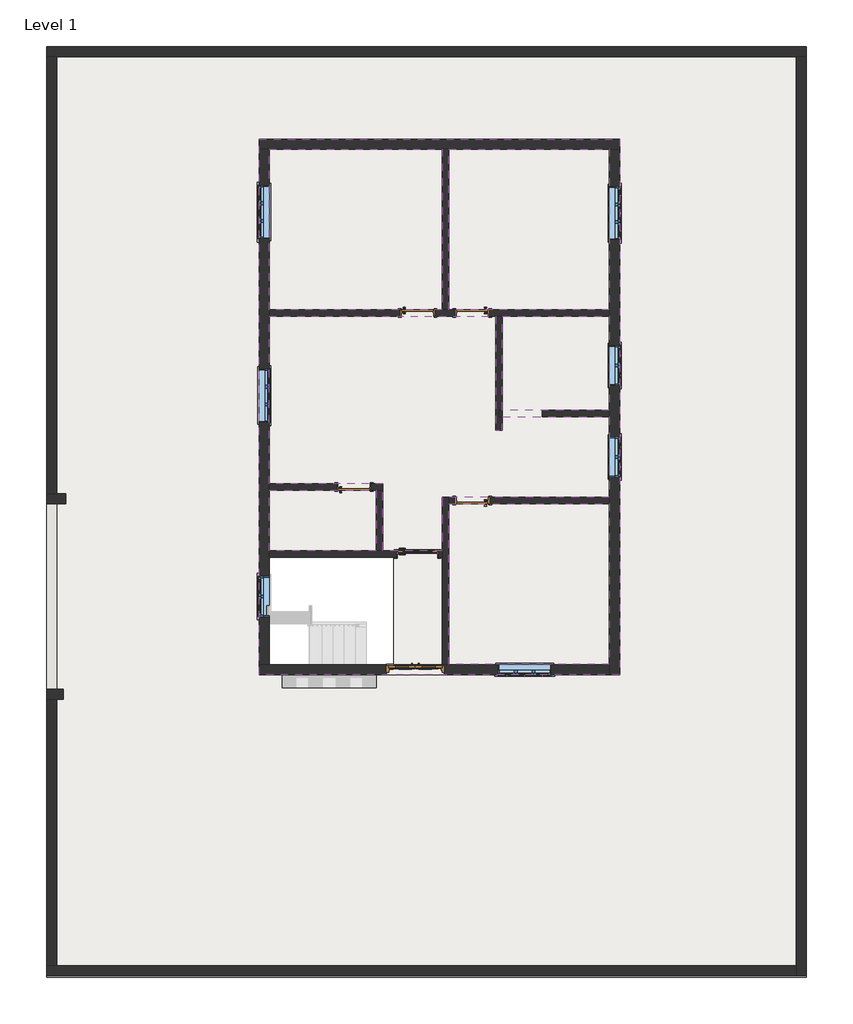
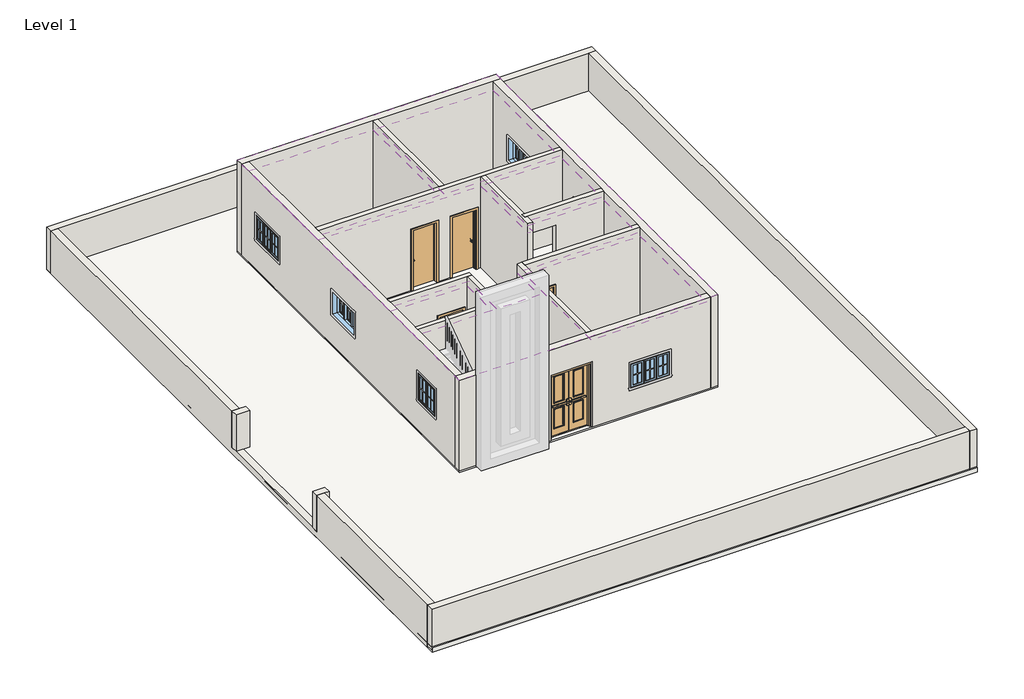
# One storey, part 1 of 2: 19 walls, 7 coverings, 7 windows, 6 doors, 2 slabs.
"""IFC4 building model written with IfcOpenShell, lengths in millimetres."""

from ifc_helpers import new_model, si_unit, frame, origin, origin_with_axes, place, context, project, spatial, polyline, outline, extrude, faceted_brep, transform, mapped, element, save
from components import door_900_x_2000mm_520166dd, m_door_exterior_double_two_lite_m_door_exterior_double_two_f203ad21, m_door_exterior_double_two_lite_m_door_exterior_double_two_3ba58653, m_door_exterior_double_two_lite_m_door_exterior_double_two_ddc6e1ea, m_door_interior_single_flush_panel_wood_m_door_interior_b00d6502, m_door_interior_single_flush_panel_wood_m_door_interior_da0777dc, m_window_awning_triple_horizontal_4_d9bc2bdd, m_window_casement_double_914_x_900mm_7ae2d64b

model = new_model("IFC4")

# Units and contexts
model_context = context("Model", 3, world=origin())
ifc_project = project(units=[si_unit("LENGTHUNIT", "METRE", prefix="MILLI")], contexts=[model_context])

# Site, building, storey
site = spatial("IfcSite", under=ifc_project)
building = spatial("IfcBuilding", under=site)
storey = spatial("IfcBuildingStorey", under=building, Name="Level 1", Elevation=0.0)

# Coverings
placement = place(None, origin())
element("IfcCovering", 1, ObjectType="2' x 4' ACT System", at=placement, inside=storey, context=model_context, shape_type="SweptSolid", body=[
    extrude(outline(polyline([(-5540.3879317, 5952.5311437), (-1603.3879317, 5952.5311437), (-1603.3879317, 2294.9311437), (-5540.3879317, 2294.9311437), (-5540.3879317, 5952.5311437)])), frame((0.0, 0.0, 2743.2), z_axis=(0.0, 0.0, 1.0), x_axis=(1.0, 0.0, 0.0)), (0.0, 0.0, 1.0), 57.15),
])
element("IfcCovering", 2, ObjectType="2' x 4' ACT System", at=placement, inside=storey, context=model_context, shape_type="SweptSolid", body=[
    extrude(outline(polyline([(-1450.9879317, 2294.9311437), (-1450.9879317, 5952.5311437), (2206.6120683, 5952.5311437), (2206.6120683, 2294.9311437), (-1450.9879317, 2294.9311437)])), frame((0.0, 0.0, 2743.2), z_axis=(0.0, 0.0, 1.0), x_axis=(1.0, 0.0, 0.0)), (0.0, 0.0, 1.0), 57.15),
])
element("IfcCovering", 3, ObjectType="2' x 4' ACT System", at=placement, inside=storey, context=model_context, shape_type="SweptSolid", body=[
    extrude(outline(polyline([(-231.7879317, -143.4688563), (2206.6120683, -143.4688563), (2206.6120683, -1972.2688563), (-1603.3879317, -1972.2688563), (-1603.3879317, -3191.4688563), (-2949.5879317, -3191.4688563), (-2949.5879317, -1667.4688563), (-5540.3879317, -1667.4688563), (-5540.3879317, 2142.5311437), (-384.1879317, 2142.5311437), (-384.1879317, -448.2688563), (-231.7879317, -448.2688563), (-231.7879317, -143.4688563)])), frame((0.0, 0.0, 2743.2), z_axis=(0.0, 0.0, 1.0), x_axis=(1.0, 0.0, 0.0)), (0.0, 0.0, 1.0), 57.15),
])
element("IfcCovering", 4, ObjectType="2' x 4' ACT System", at=placement, inside=storey, context=model_context, shape_type="SweptSolid", body=[
    extrude(outline(polyline([(2206.6120683, 2142.5311437), (2206.6120683, 8.9311437), (-231.7879317, 8.9311437), (-231.7879317, 2142.5311437), (2206.6120683, 2142.5311437)])), frame((0.0, 0.0, 2743.2), z_axis=(0.0, 0.0, 1.0), x_axis=(1.0, 0.0, 0.0)), (0.0, 0.0, 1.0), 57.15),
])
element("IfcCovering", 5, ObjectType="2' x 4' ACT System", at=placement, inside=storey, context=model_context, shape_type="SweptSolid", body=[
    extrude(outline(polyline([(-3101.9879317, -3191.4688563), (-5540.3879317, -3191.4688563), (-5540.3879317, -1819.8688563), (-3101.9879317, -1819.8688563), (-3101.9879317, -3191.4688563)])), frame((0.0, 0.0, 2743.2), z_axis=(0.0, 0.0, 1.0), x_axis=(1.0, 0.0, 0.0)), (0.0, 0.0, 1.0), 57.15),
])
element("IfcCovering", 6, ObjectType="2' x 4' ACT System", at=placement, inside=storey, context=model_context, shape_type="SweptSolid", body=[
    extrude(outline(polyline([(2206.6120683, -2124.6688563), (2206.6120683, -5782.2688563), (-1450.9879317, -5782.2688563), (-1450.9879317, -2124.6688563), (2206.6120683, -2124.6688563)])), frame((0.0, 0.0, 2743.2), z_axis=(0.0, 0.0, 1.0), x_axis=(1.0, 0.0, 0.0)), (0.0, 0.0, 1.0), 57.15),
])
element("IfcCovering", 7, ObjectType="2' x 4' ACT System", at=placement, inside=storey, context=model_context, shape_type="SweptSolid", body=[
    extrude(outline(polyline([(-5768.9879317, 6181.1311437), (2435.2120683, 6181.1311437), (2435.2120683, -6010.8688563), (-5768.9879317, -6010.8688563), (-5768.9879317, 6181.1311437)]), holes=[polyline([(-5540.3879317, -3343.8688563), (-5540.3879317, -5895.1313563), (-2720.1879317, -5895.1313563), (-2720.1879317, -5782.2688563), (-2720.1879317, -4715.4688563), (-2720.1879317, -3343.8688563), (-4130.2879317, -3343.8688563), (-5540.3879317, -3343.8688563)])]), frame((0.0, 0.0, 3048.0), z_axis=(0.0, 0.0, 1.0), x_axis=(1.0, 0.0, 0.0)), (0.0, 0.0, 1.0), 57.15),
])

# Doors
door_900_x_2000mm_shape = door_900_x_2000mm_520166dd(model_context)
element("IfcDoor", 8, ObjectType="900 x 2000mm", at=placement, inside=storey, context=model_context, shape_type="MappedRepresentation", body=[
    mapped(door_900_x_2000mm_shape, transform((-2162.1879317, -3264.4938563, 0.0), x_axis=(-1.0, 0.0, 0.0), y_axis=(0.0, -1.0, 0.0), z_axis=(0.0, 0.0, 1.0))),
])
m_door_exterior_double_two_lite_m_door_exterior_double_two_shape = m_door_exterior_double_two_lite_m_door_exterior_double_two_f203ad21(model_context)
m_door_exterior_double_two_lite_m_door_exterior_double_two_2_shape = m_door_exterior_double_two_lite_m_door_exterior_double_two_3ba58653(model_context)
m_door_exterior_double_two_lite_m_door_exterior_double_two_3_shape = m_door_exterior_double_two_lite_m_door_exterior_double_two_ddc6e1ea(model_context)
element("IfcDoor", 9, ObjectType="M_Door-Exterior-Double-Two_Lite : M_Door-Exterior-Double-Two_Lite", at=placement, inside=storey, context=model_context, shape_type="MappedRepresentation", body=[
    mapped(m_door_exterior_double_two_lite_m_door_exterior_double_two_shape, transform((-2212.9879317, -5902.9188563, 0.0), x_axis=(1.0, 0.0, 0.0), y_axis=(0.0, 1.0, 0.0), z_axis=(0.0, 0.0, 1.0))),
    mapped(m_door_exterior_double_two_lite_m_door_exterior_double_two_2_shape, transform((-2212.9879317, -5902.9188563, 0.0), x_axis=(1.0, 0.0, 0.0), y_axis=(0.0, 1.0, 0.0), z_axis=(0.0, 0.0, 1.0))),
    mapped(m_door_exterior_double_two_lite_m_door_exterior_double_two_3_shape, transform((-2212.9879317, -5902.9188563, 0.0), x_axis=(1.0, 0.0, 0.0), y_axis=(0.0, 1.0, 0.0), z_axis=(0.0, 0.0, 1.0))),
])
m_door_interior_single_flush_panel_wood_m_door_interior_shape = m_door_interior_single_flush_panel_wood_m_door_interior_b00d6502(model_context)
element("IfcDoor", 10, ObjectType="M_Door-Interior-Single-Flush_Panel-Wood : M_Door-Interior-Single-Flush_Panel-Wood", at=placement, inside=storey, context=model_context, shape_type="MappedRepresentation", body=[
    mapped(m_door_interior_single_flush_panel_wood_m_door_interior_shape, transform((-3609.9879317, -1746.8438563, 0.0), x_axis=(1.0, 0.0, 0.0), y_axis=(0.0, 1.0, 0.0), z_axis=(0.0, 0.0, 1.0))),
])
element("IfcDoor", 11, ObjectType="M_Door-Interior-Single-Flush_Panel-Wood : M_Door-Interior-Single-Flush_Panel-Wood", at=placement, inside=storey, context=model_context, shape_type="MappedRepresentation", body=[
    mapped(m_door_interior_single_flush_panel_wood_m_door_interior_shape, transform((-917.5879317, 2221.9061437, 0.0), x_axis=(-1.0, 0.0, 0.0), y_axis=(0.0, -1.0, 0.0), z_axis=(0.0, 0.0, 1.0))),
])
m_door_interior_single_flush_panel_wood_m_door_interior_2_shape = m_door_interior_single_flush_panel_wood_m_door_interior_da0777dc(model_context)
element("IfcDoor", 12, ObjectType="M_Door-Interior-Single-Flush_Panel-Wood : M_Door-Interior-Single-Flush_Panel-Wood", at=placement, inside=storey, context=model_context, shape_type="MappedRepresentation", body=[
    mapped(m_door_interior_single_flush_panel_wood_m_door_interior_2_shape, transform((-917.5879317, -2051.6438563, 0.0), x_axis=(-1.0, 0.0, 0.0), y_axis=(0.0, -1.0, 0.0), z_axis=(0.0, 0.0, 1.0))),
])
element("IfcDoor", 13, ObjectType="M_Door-Interior-Single-Flush_Panel-Wood : M_Door-Interior-Single-Flush_Panel-Wood", at=placement, inside=storey, context=model_context, shape_type="MappedRepresentation", body=[
    mapped(m_door_interior_single_flush_panel_wood_m_door_interior_2_shape, transform((-2162.1879317, 2221.9061437, 0.0), x_axis=(1.0, 0.0, 0.0), y_axis=(0.0, 1.0, 0.0), z_axis=(0.0, 0.0, 1.0))),
])

# Slabs
element("IfcSlab", 14, ObjectType="Generic - 6\"", at=placement, inside=storey, context=model_context, shape_type="SweptSolid", body=[
    extrude(outline(polyline([(-5768.9879317, -6010.8688563), (-5768.9879317, 6181.1311437), (2435.2120683, 6181.1311437), (2435.2120683, -6010.8688563), (-5768.9879317, -6010.8688563)]), holes=[polyline([(-5540.3879317, -3343.8688563), (-5540.3879317, -5895.1313563), (-2720.1879317, -5895.1313563), (-2720.1879317, -5782.2688563), (-2720.1879317, -4715.4688563), (-2720.1879317, -3343.8688563), (-4130.2879317, -3343.8688563), (-5540.3879317, -3343.8688563)])]), frame((0.0, 0.0, -152.4), z_axis=(0.0, 0.0, 1.0), x_axis=(1.0, 0.0, 0.0)), (0.0, 0.0, 1.0), 152.4),
])
element("IfcSlab", 15, ObjectType="Generic - 6\"", at=placement, inside=storey, context=model_context, shape_type="SweptSolid", body=[
    extrude(outline(polyline([(-10609.2377926, -12906.9688563), (-10609.2377926, 8286.7256462), (6688.1622074, 8286.7256462), (6688.1622074, -12906.9688563), (-10609.2377926, -12906.9688563)]), holes=[polyline([(-5540.3879317, -3343.8688563), (-5540.3879317, -5895.1313563), (-2720.1879317, -5895.1313563), (-2720.1879317, -5782.2688563), (-2720.1879317, -4715.4688563), (-2720.1879317, -3343.8688563), (-4130.2879317, -3343.8688563), (-5540.3879317, -3343.8688563)])]), frame((0.0, 0.0, -203.2), z_axis=(0.0, 0.0, 1.0), x_axis=(1.0, 0.0, 0.0)), (0.0, 0.0, 1.0), 152.4),
])

# Walls
element("IfcWall", 16, ObjectType="Generic - 6\"", at=placement, inside=storey, context=model_context, shape_type="SweptSolid", body=[
    extrude(outline(polyline([(-1603.3879317, 2294.9311437), (-1603.3879317, 5952.5311437), (-1450.9879317, 5952.5311437), (-1450.9879317, 2294.9311437), (-1603.3879317, 2294.9311437)])), origin_with_axes(), (0.0, 0.0, 1.0), 3048.0),
])
element("IfcWall", 17, ObjectType="Generic - 6\"", at=placement, inside=storey, context=model_context, shape_type="Brep", body=[
    faceted_brep([(2206.6120683, 2142.5311437, 3048.0), (-231.7879317, 2142.5311437, 3048.0), (-384.1879317, 2142.5311437, 3048.0), (-5540.3879317, 2142.5311437, 3048.0), (-5540.3879317, 2142.5311437, 0.0), (-2555.4879317, 2142.5311437, 0.0), (-2555.4879317, 2142.5311437, 2025.0), (-1768.8879317, 2142.5311437, 2025.0), (-1768.8879317, 2142.5311437, 0.0), (-1310.8879317, 2142.5311437, 0.0), (-1310.8879317, 2142.5311437, 2025.0), (-524.2879317, 2142.5311437, 2025.0), (-524.2879317, 2142.5311437, 0.0), (-384.1879317, 2142.5311437, 0.0), (-231.7879317, 2142.5311437, 0.0), (2206.6120683, 2142.5311437, 0.0), (-5540.3879317, 2294.9311437, 3048.0), (-1603.3879317, 2294.9311437, 3048.0), (-1450.9879317, 2294.9311437, 3048.0), (2206.6120683, 2294.9311437, 3048.0), (2206.6120683, 2294.9311437, 0.0), (-524.2879317, 2294.9311437, 0.0), (-524.2879317, 2294.9311437, 2025.0), (-1310.8879317, 2294.9311437, 2025.0), (-1310.8879317, 2294.9311437, 0.0), (-1450.9879317, 2294.9311437, 0.0), (-1603.3879317, 2294.9311437, 0.0), (-1768.8879317, 2294.9311437, 0.0), (-1768.8879317, 2294.9311437, 2025.0), (-2555.4879317, 2294.9311437, 2025.0), (-2555.4879317, 2294.9311437, 0.0), (-5540.3879317, 2294.9311437, 0.0)], [[[0, 1, 2, 3, 4, 5, 6, 7, 8, 9, 10, 11, 12, 13, 14, 15]], [[16, 17, 18, 19, 20, 21, 22, 23, 24, 25, 26, 27, 28, 29, 30, 31]], [[4, 31, 30, 5]], [[20, 15, 14, 13, 12, 21]], [[8, 27, 26, 25, 24, 9]], [[3, 2, 1, 0, 19, 18, 17, 16]], [[0, 15, 20, 19]], [[4, 3, 16, 31]], [[7, 28, 27, 8]], [[28, 7, 6, 29]], [[29, 6, 5, 30]], [[23, 10, 9, 24]], [[10, 23, 22, 11]], [[11, 22, 21, 12]]]),
])
element("IfcWall", 18, ObjectType="Generic - 6\"", at=placement, inside=storey, context=model_context, shape_type="SweptSolid", body=[
    extrude(outline(polyline([(-384.1879317, -448.2688563), (-384.1879317, 2142.5311437), (-231.7879317, 2142.5311437), (-231.7879317, -448.2688563), (-384.1879317, -448.2688563)])), origin_with_axes(), (0.0, 0.0, 1.0), 3048.0),
])
element("IfcWall", 19, ObjectType="Generic - 6\"", at=placement, inside=storey, context=model_context, shape_type="SweptSolid", body=[
    extrude(outline(polyline([(3048.0, -307.9879317), (0.0, -307.9879317), (0.0, -234.2341596), (2438.4, -234.2341596), (2438.4, 675.543661), (0.0, 675.543661), (0.0, 2206.6120683), (3048.0, 2206.6120683), (3048.0, -307.9879317)])), frame((0.0, -143.4688563, 0.0), z_axis=(0.0, 1.0, 0.0), x_axis=(0.0, 0.0, 1.0)), (0.0, 0.0, 1.0), 152.4),
])
element("IfcWall", 20, ObjectType="Generic - 6\"", at=placement, inside=storey, context=model_context, shape_type="Brep", body=[
    faceted_brep([(-2949.5879317, -1819.8688563, 3048.0), (-3101.9879317, -1819.8688563, 3048.0), (-5540.3879317, -1819.8688563, 3048.0), (-5540.3879317, -1819.8688563, 0.0), (-4003.2879317, -1819.8688563, 0.0), (-4003.2879317, -1819.8688563, 2025.0), (-3216.6879317, -1819.8688563, 2025.0), (-3216.6879317, -1819.8688563, 0.0), (-3101.9879317, -1819.8688563, 0.0), (-2949.5879317, -1819.8688563, 0.0), (-5540.3879317, -1667.4688563, 3048.0), (-2949.5879317, -1667.4688563, 3048.0), (-2949.5879317, -1667.4688563, 0.0), (-3216.6879317, -1667.4688563, 0.0), (-3216.6879317, -1667.4688563, 2025.0), (-4003.2879317, -1667.4688563, 2025.0), (-4003.2879317, -1667.4688563, 0.0), (-5540.3879317, -1667.4688563, 0.0)], [[[0, 1, 2, 3, 4, 5, 6, 7, 8, 9]], [[10, 11, 12, 13, 14, 15, 16, 17]], [[3, 17, 16, 4]], [[12, 9, 8, 7, 13]], [[2, 1, 0, 11, 10]], [[3, 2, 10, 17]], [[0, 9, 12, 11]], [[6, 14, 13, 7]], [[14, 6, 5, 15]], [[15, 5, 4, 16]]]),
])
element("IfcWall", 21, ObjectType="Generic - 6\"", at=placement, inside=storey, context=model_context, shape_type="SweptSolid", body=[
    extrude(outline(polyline([(-3101.9879317, -3191.4688563), (-3101.9879317, -1819.8688563), (-2949.5879317, -1819.8688563), (-2949.5879317, -3191.4688563), (-3101.9879317, -3191.4688563)])), origin_with_axes(), (0.0, 0.0, 1.0), 3048.0),
])
element("IfcWall", 22, ObjectType="Generic - 6\"", at=placement, inside=storey, context=model_context, shape_type="Brep", body=[
    faceted_brep([(-1603.3879317, -3343.8688563, 3048.0), (-5540.3879317, -3343.8688563, 3048.0), (-5540.3879317, -3343.8688563, 0.0), (-2644.3879317, -3343.8688563, 0.0), (-2644.3879317, -3343.8688563, 2025.0), (-1679.9879317, -3343.8688563, 2025.0), (-1679.9879317, -3343.8688563, 0.0), (-1603.3879317, -3343.8688563, 0.0), (-5540.3879317, -3191.4688563, 3048.0), (-3101.9879317, -3191.4688563, 3048.0), (-2949.5879317, -3191.4688563, 3048.0), (-1603.3879317, -3191.4688563, 3048.0), (-1603.3879317, -3191.4688563, 0.0), (-1679.9879317, -3191.4688563, 0.0), (-1679.9879317, -3191.4688563, 2025.0), (-2644.3879317, -3191.4688563, 2025.0), (-2644.3879317, -3191.4688563, 0.0), (-2949.5879317, -3191.4688563, 0.0), (-3101.9879317, -3191.4688563, 0.0), (-5540.3879317, -3191.4688563, 0.0)], [[[0, 1, 2, 3, 4, 5, 6, 7]], [[8, 9, 10, 11, 12, 13, 14, 15, 16, 17, 18, 19]], [[2, 19, 18, 17, 16, 3]], [[12, 7, 6, 13]], [[1, 0, 11, 10, 9, 8]], [[2, 1, 8, 19]], [[0, 7, 12, 11]], [[15, 4, 3, 16]], [[4, 15, 14, 5]], [[5, 14, 13, 6]]]),
])
element("IfcWall", 23, ObjectType="Generic - 6\"", at=placement, inside=storey, context=model_context, shape_type="Brep", body=[
    faceted_brep([(-1450.9879317, -5782.2688563, 0.0), (-1450.9879317, -2124.6688563, 0.0), (-1450.9879317, -1972.2688563, 0.0), (-1450.9879317, -1972.2688563, 3048.0), (-1450.9879317, -2124.6688563, 3048.0), (-1450.9879317, -5782.2688563, 3048.0), (-1603.3879317, -5782.2688563, 0.0), (-1603.3879317, -5782.2688563, 3048.0), (-1603.3879317, -3343.8688563, 3048.0), (-1603.3879317, -3191.4688563, 3048.0), (-1603.3879317, -1972.2688563, 3048.0), (-1603.3879317, -1972.2688563, 0.0), (-1603.3879317, -3191.4688563, 0.0), (-1603.3879317, -3343.8688563, 0.0)], [[[0, 1, 2, 3, 4, 5]], [[6, 7, 8, 9, 10, 11, 12, 13]], [[2, 1, 0, 6, 13, 12, 11]], [[5, 4, 3, 10, 9, 8, 7]], [[0, 5, 7, 6]], [[3, 2, 11, 10]]]),
])
element("IfcWall", 24, ObjectType="Generic - 6\"", at=placement, inside=storey, context=model_context, shape_type="SweptSolid", body=[
    extrude(outline(polyline([(3048.0, 2206.6120683), (3048.0, -1450.9879317), (0.0, -1450.9879317), (0.0, -1310.8879317), (2025.0, -1310.8879317), (2025.0, -524.2879317), (0.0, -524.2879317), (0.0, 2206.6120683), (3048.0, 2206.6120683)])), frame((0.0, -2124.6688563, 0.0), z_axis=(0.0, 1.0, 0.0), x_axis=(0.0, 0.0, 1.0)), (0.0, 0.0, 1.0), 152.4),
])
element("IfcWall", 25, ObjectType="Generic - 9\"", at=placement, inside=storey, context=model_context, shape_type="Brep", body=[
    faceted_brep([(-5768.9879317, 5952.5311437, 0.0), (-5540.3879317, 5952.5311437, 0.0), (-1603.3879317, 5952.5311437, 0.0), (-1450.9879317, 5952.5311437, 0.0), (2206.6120683, 5952.5311437, 0.0), (2435.2120683, 5952.5311437, 0.0), (2435.2120683, 5952.5311437, 3048.0), (2206.6120683, 5952.5311437, 3048.0), (-1450.9879317, 5952.5311437, 3048.0), (-1603.3879317, 5952.5311437, 3048.0), (-5540.3879317, 5952.5311437, 3048.0), (-5768.9879317, 5952.5311437, 3048.0), (-5768.9879317, 6181.1311437, 0.0), (-5768.9879317, 6181.1311437, 3048.0), (2435.2120683, 6181.1311437, 3048.0), (2435.2120683, 6181.1311437, 0.0)], [[[0, 1, 2, 3, 4, 5, 6, 7, 8, 9, 10, 11]], [[12, 13, 14, 15]], [[5, 4, 3, 2, 1, 0, 12, 15]], [[11, 10, 9, 8, 7, 6, 14, 13]], [[6, 5, 15, 14]], [[0, 11, 13, 12]]]),
])
element("IfcWall", 26, ObjectType="Generic - 9\"", at=placement, inside=storey, context=model_context, shape_type="Brep", body=[
    faceted_brep([(2206.6120683, 5952.5311437, 0.0), (2206.6120683, 2294.9311437, 0.0), (2206.6120683, 2142.5311437, 0.0), (2206.6120683, 8.9311437, 0.0), (2206.6120683, -143.4688563, 0.0), (2206.6120683, -1972.2688563, 0.0), (2206.6120683, -2124.6688563, 0.0), (2206.6120683, -5782.2688563, 0.0), (2206.6120683, -6010.8688563, 0.0), (2206.6120683, -6010.8688563, 3048.0), (2206.6120683, -5782.2688563, 3048.0), (2206.6120683, -2124.6688563, 3048.0), (2206.6120683, -1972.2688563, 3048.0), (2206.6120683, -143.4688563, 3048.0), (2206.6120683, 8.9311437, 3048.0), (2206.6120683, 2142.5311437, 3048.0), (2206.6120683, 2294.9311437, 3048.0), (2206.6120683, 5952.5311437, 3048.0), (2206.6120683, 3882.4311437, 1700.0), (2206.6120683, 3882.4311437, 900.0), (2206.6120683, 5101.6311437, 900.0), (2206.6120683, 5101.6311437, 1700.0), (2206.6120683, -1515.0688563, 1800.0), (2206.6120683, -1515.0688563, 900.0), (2206.6120683, -600.6688563, 900.0), (2206.6120683, -600.6688563, 1800.0), (2206.6120683, 567.7311437, 1800.0), (2206.6120683, 567.7311437, 900.0), (2206.6120683, 1482.1311437, 900.0), (2206.6120683, 1482.1311437, 1800.0), (2435.2120683, 5952.5311437, 0.0), (2435.2120683, 5952.5311437, 3048.0), (2435.2120683, -6010.8688563, 3048.0), (2435.2120683, -6010.8688563, 0.0), (2435.2120683, 3882.4311437, 1700.0), (2435.2120683, 5101.6311437, 1700.0), (2435.2120683, 5101.6311437, 900.0), (2435.2120683, 3882.4311437, 900.0), (2435.2120683, -1515.0688563, 1800.0), (2435.2120683, -600.6688563, 1800.0), (2435.2120683, -600.6688563, 900.0), (2435.2120683, -1515.0688563, 900.0), (2435.2120683, 567.7311437, 1800.0), (2435.2120683, 1482.1311437, 1800.0), (2435.2120683, 1482.1311437, 900.0), (2435.2120683, 567.7311437, 900.0)], [[[0, 1, 2, 3, 4, 5, 6, 7, 8, 9, 10, 11, 12, 13, 14, 15, 16, 17], [18, 19, 20, 21], [22, 23, 24, 25], [26, 27, 28, 29]], [[30, 31, 32, 33], [34, 35, 36, 37], [38, 39, 40, 41], [42, 43, 44, 45]], [[8, 7, 6, 5, 4, 3, 2, 1, 0, 30, 33]], [[17, 16, 15, 14, 13, 12, 11, 10, 9, 32, 31]], [[0, 17, 31, 30]], [[9, 8, 33, 32]], [[19, 18, 34, 37]], [[20, 19, 37, 36]], [[21, 20, 36, 35]], [[18, 21, 35, 34]], [[23, 22, 38, 41]], [[24, 23, 41, 40]], [[25, 24, 40, 39]], [[22, 25, 39, 38]], [[27, 26, 42, 45]], [[28, 27, 45, 44]], [[29, 28, 44, 43]], [[26, 29, 43, 42]]]),
])
element("IfcWall", 27, ObjectType="Generic - 9\"", at=placement, inside=storey, context=model_context, shape_type="Brep", body=[
    faceted_brep([(-5768.9879317, -5782.2688563, 3048.0), (-5540.3879317, -5782.2688563, 3048.0), (-1603.3879317, -5782.2688563, 3048.0), (-1450.9879317, -5782.2688563, 3048.0), (2206.6120683, -5782.2688563, 3048.0), (2206.6120683, -5782.2688563, 0.0), (-1450.9879317, -5782.2688563, 0.0), (-1553.3879317, -5782.2688563, 0.0), (-1553.3879317, -5782.2688563, 2200.0), (-2872.5879317, -5782.2688563, 2200.0), (-2872.5879317, -5782.2688563, 0.0), (-5540.3879317, -5782.2688563, 0.0), (-5768.9879317, -5782.2688563, 0.0), (-333.3879317, -5782.2688563, 1700.0), (-333.3879317, -5782.2688563, 900.0), (885.8120683, -5782.2688563, 900.0), (885.8120683, -5782.2688563, 1700.0), (2206.6120683, -6010.8688563, 3048.0), (-5768.9879317, -6010.8688563, 3048.0), (-5768.9879317, -6010.8688563, 0.0), (-2872.5879317, -6010.8688563, 0.0), (-2872.5879317, -6010.8688563, 2200.0), (-1553.3879317, -6010.8688563, 2200.0), (-1553.3879317, -6010.8688563, 0.0), (2206.6120683, -6010.8688563, 0.0), (-333.3879317, -6010.8688563, 1700.0), (885.8120683, -6010.8688563, 1700.0), (885.8120683, -6010.8688563, 900.0), (-333.3879317, -6010.8688563, 900.0)], [[[0, 1, 2, 3, 4, 5, 6, 7, 8, 9, 10, 11, 12], [13, 14, 15, 16]], [[17, 18, 19, 20, 21, 22, 23, 24], [25, 26, 27, 28]], [[5, 24, 23, 7, 6]], [[19, 12, 11, 10, 20]], [[4, 3, 2, 1, 0, 18, 17]], [[5, 4, 17, 24]], [[0, 12, 19, 18]], [[22, 8, 7, 23]], [[8, 22, 21, 9]], [[9, 21, 20, 10]], [[14, 13, 25, 28]], [[15, 14, 28, 27]], [[16, 15, 27, 26]], [[13, 16, 26, 25]]]),
])
element("IfcWall", 28, ObjectType="Generic - 9\"", at=placement, inside=storey, context=model_context, shape_type="Brep", body=[
    faceted_brep([(-5540.3879317, -5782.2688563, 0.0), (-5540.3879317, -3343.8688563, 0.0), (-5540.3879317, -3191.4688563, 0.0), (-5540.3879317, -1819.8688563, 0.0), (-5540.3879317, -1667.4688563, 0.0), (-5540.3879317, 2142.5311437, 0.0), (-5540.3879317, 2294.9311437, 0.0), (-5540.3879317, 5952.5311437, 0.0), (-5540.3879317, 5952.5311437, 3048.0), (-5540.3879317, 2294.9311437, 3048.0), (-5540.3879317, 2142.5311437, 3048.0), (-5540.3879317, -1667.4688563, 3048.0), (-5540.3879317, -1819.8688563, 3048.0), (-5540.3879317, -3191.4688563, 3048.0), (-5540.3879317, -3343.8688563, 3048.0), (-5540.3879317, -5782.2688563, 3048.0), (-5540.3879317, 5127.0311437, 1841.4), (-5540.3879317, 5127.0311437, 1041.4), (-5540.3879317, 3907.8311437, 1041.4), (-5540.3879317, 3907.8311437, 1841.4), (-5540.3879317, -270.4688563, 1841.4), (-5540.3879317, 948.7311437, 1841.4), (-5540.3879317, 948.7311437, 1041.4), (-5540.3879317, -270.4688563, 1041.4), (-5540.3879317, -3775.6688563, 1941.4), (-5540.3879317, -3775.6688563, 1041.4), (-5540.3879317, -4690.0688563, 1041.4), (-5540.3879317, -4690.0688563, 1941.4), (-5768.9879317, -5782.2688563, 0.0), (-5768.9879317, -5782.2688563, 3048.0), (-5768.9879317, 5952.5311437, 3048.0), (-5768.9879317, 5952.5311437, 0.0), (-5768.9879317, 5127.0311437, 1841.4), (-5768.9879317, 3907.8311437, 1841.4), (-5768.9879317, 3907.8311437, 1041.4), (-5768.9879317, 5127.0311437, 1041.4), (-5768.9879317, -270.4688563, 1841.4), (-5768.9879317, -270.4688563, 1041.4), (-5768.9879317, 948.7311437, 1041.4), (-5768.9879317, 948.7311437, 1841.4), (-5768.9879317, -3775.6688563, 1941.4), (-5768.9879317, -4690.0688563, 1941.4), (-5768.9879317, -4690.0688563, 1041.4), (-5768.9879317, -3775.6688563, 1041.4)], [[[0, 1, 2, 3, 4, 5, 6, 7, 8, 9, 10, 11, 12, 13, 14, 15], [16, 17, 18, 19], [20, 21, 22, 23], [24, 25, 26, 27]], [[28, 29, 30, 31], [32, 33, 34, 35], [36, 37, 38, 39], [40, 41, 42, 43]], [[7, 6, 5, 4, 3, 2, 1, 0, 28, 31]], [[15, 14, 13, 12, 11, 10, 9, 8, 30, 29]], [[8, 7, 31, 30]], [[0, 15, 29, 28]], [[17, 16, 32, 35]], [[18, 17, 35, 34]], [[19, 18, 34, 33]], [[16, 19, 33, 32]], [[37, 36, 20, 23]], [[38, 37, 23, 22]], [[39, 38, 22, 21]], [[36, 39, 21, 20]], [[25, 24, 40, 43]], [[26, 25, 43, 42]], [[27, 26, 42, 41]], [[24, 27, 41, 40]]]),
])
element("IfcWall", 29, ObjectType="Generic - 9\"", at=placement, inside=storey, context=model_context, shape_type="Brep", body=[
    faceted_brep([(-10609.2377926, 8058.1256462, -188.2211546), (6688.1622074, 8058.1256462, -188.2211546), (6688.1622074, 8058.1256462, 1219.2), (6459.5622074, 8058.1256462, 1219.2), (-10380.6377926, 8058.1256462, 1219.2), (-10609.2377926, 8058.1256462, 1219.2), (-10609.2377926, 8286.7256462, -188.2211546), (-10609.2377926, 8286.7256462, 1219.2), (6688.1622074, 8286.7256462, 1219.2), (6688.1622074, 8286.7256462, -188.2211546)], [[[0, 1, 2, 3, 4, 5]], [[6, 7, 8, 9]], [[1, 0, 6, 9]], [[5, 4, 3, 2, 8, 7]], [[2, 1, 9, 8]], [[0, 5, 7, 6]]]),
])
element("IfcWall", 30, ObjectType="Generic - 9\"", at=placement, inside=storey, context=model_context, shape_type="Brep", body=[
    faceted_brep([(6459.5622074, 8058.1256462, -207.0200215), (6459.5622074, -12868.8688563, -207.0200215), (6459.5622074, -12868.8688563, -152.4), (6459.5622074, -12868.8688563, 1219.2), (6459.5622074, -12640.2688563, 1219.2), (6459.5622074, 8058.1256462, 1219.2), (6688.1622074, 8058.1256462, -207.0200215), (6688.1622074, 8058.1256462, -188.2211546), (6688.1622074, 8058.1256462, 1219.2), (6688.1622074, -12868.8688563, 1219.2), (6688.1622074, -12868.8688563, -207.0200215)], [[[0, 1, 2, 3, 4, 5]], [[6, 7, 8, 9, 10]], [[1, 0, 6, 10]], [[5, 4, 3, 9, 8]], [[0, 5, 8, 7, 6]], [[3, 2, 1, 10, 9]]]),
])
element("IfcWall", 31, ObjectType="Generic - 9\"", at=placement, inside=storey, context=model_context, shape_type="Brep", body=[
    faceted_brep([(6459.5622074, -12640.2688563, -152.4), (-10609.2377926, -12640.2688563, -152.4), (-10609.2377926, -12640.2688563, 1219.2), (-10380.6377926, -12640.2688563, 1219.2), (6459.5622074, -12640.2688563, 1219.2), (6459.5622074, -12868.8688563, -152.4), (6459.5622074, -12868.8688563, 1219.2), (-10609.2377926, -12868.8688563, 1219.2), (-10609.2377926, -12868.8688563, -152.4)], [[[0, 1, 2, 3, 4]], [[5, 6, 7, 8]], [[1, 0, 5, 8]], [[4, 3, 2, 7, 6]], [[0, 4, 6, 5]], [[2, 1, 8, 7]]]),
])
element("IfcWall", 32, ObjectType="Generic - 9\"", at=placement, inside=storey, context=model_context, shape_type="Brep", body=[
    faceted_brep([(-10380.6377926, -12640.2688563, -203.2), (-10380.6377926, 8058.1256462, -203.2), (-10380.6377926, 8058.1256462, 1219.2), (-10380.6377926, -1899.0730187, 1219.2), (-10380.6377926, -1899.0730187, 0.0), (-10380.6377926, -6574.4484417, 0.0), (-10380.6377926, -6574.4484417, 1219.2), (-10380.6377926, -12640.2688563, 1219.2), (-10609.2377926, 8058.1256462, -203.2), (-10609.2377926, -12640.2688563, -203.2), (-10609.2377926, -12640.2688563, -152.4), (-10609.2377926, -12640.2688563, 1219.2), (-10609.2377926, -6574.4484417, 1219.2), (-10609.2377926, -6574.4484417, 0.0), (-10609.2377926, -6345.8484417, 0.0), (-10609.2377926, -2127.6730187, 0.0), (-10609.2377926, -1899.0730187, 0.0), (-10609.2377926, -1899.0730187, 1219.2), (-10609.2377926, 8058.1256462, 1219.2), (-10609.2377926, 8058.1256462, -188.2211546)], [[[0, 1, 2, 3, 4, 5, 6, 7]], [[8, 9, 10, 11, 12, 13, 14, 15, 16, 17, 18, 19]], [[1, 0, 9, 8]], [[11, 7, 6, 12]], [[2, 18, 17, 3]], [[2, 1, 8, 19, 18]], [[0, 7, 11, 10, 9]], [[4, 16, 15, 14, 13, 5]], [[5, 13, 12, 6]], [[16, 4, 3, 17]]]),
])
element("IfcWall", 33, ObjectType="Generic - 9\"", at=placement, inside=storey, context=model_context, shape_type="Brep", body=[
    faceted_brep([(-10609.2377926, -6574.4484417, 0.0), (-10380.6377926, -6574.4484417, 0.0), (-10228.2377926, -6574.4484417, 0.0), (-10228.2377926, -6574.4484417, 1219.2), (-10380.6377926, -6574.4484417, 1219.2), (-10609.2377926, -6574.4484417, 1219.2), (-10609.2377926, -6345.8484417, 0.0), (-10609.2377926, -6345.8484417, 1219.2), (-10228.2377926, -6345.8484417, 1219.2), (-10228.2377926, -6345.8484417, 0.0)], [[[0, 1, 2, 3, 4, 5]], [[6, 7, 8, 9]], [[2, 1, 0, 6, 9]], [[3, 2, 9, 8]], [[5, 4, 3, 8, 7]], [[0, 5, 7, 6]]]),
])
element("IfcWall", 34, ObjectType="Generic - 9\"", at=placement, inside=storey, context=model_context, shape_type="Brep", body=[
    faceted_brep([(-10609.2377926, -2127.6730187, 0.0), (-10177.4377926, -2127.6730187, 0.0), (-10177.4377926, -2127.6730187, 1219.2), (-10609.2377926, -2127.6730187, 1219.2), (-10609.2377926, -1899.0730187, 0.0), (-10609.2377926, -1899.0730187, 1219.2), (-10380.6377926, -1899.0730187, 1219.2), (-10177.4377926, -1899.0730187, 1219.2), (-10177.4377926, -1899.0730187, 0.0), (-10380.6377926, -1899.0730187, 0.0)], [[[0, 1, 2, 3]], [[4, 5, 6, 7, 8, 9]], [[1, 0, 4, 9, 8]], [[2, 1, 8, 7]], [[3, 2, 7, 6, 5]], [[0, 3, 5, 4]]]),
])

# Windows
m_window_awning_triple_horizontal_4_shape = m_window_awning_triple_horizontal_4_d9bc2bdd(model_context)
element("IfcWindow", 35, ObjectType="M_Window-Awning-Triple-Horizontal : 4'", at=placement, inside=storey, context=model_context, shape_type="MappedRepresentation", body=[
    mapped(m_window_awning_triple_horizontal_4_shape, transform((-5654.6879317, 4517.4311437, 141.4), x_axis=(0.0, 1.0, 0.0), y_axis=(-1.0, 0.0, 0.0), z_axis=(0.0, 0.0, 1.0))),
])
element("IfcWindow", 36, ObjectType="M_Window-Awning-Triple-Horizontal : 4'", at=placement, inside=storey, context=model_context, shape_type="MappedRepresentation", body=[
    mapped(m_window_awning_triple_horizontal_4_shape, transform((2320.9120683, 4492.0311437, 0.0), x_axis=(0.0, -1.0, 0.0), y_axis=(1.0, 0.0, 0.0), z_axis=(0.0, 0.0, 1.0))),
])
element("IfcWindow", 37, ObjectType="M_Window-Awning-Triple-Horizontal : 4'", at=placement, inside=storey, context=model_context, shape_type="MappedRepresentation", body=[
    mapped(m_window_awning_triple_horizontal_4_shape, transform((-5654.6879317, 339.1311437, 141.4), x_axis=(0.0, -1.0, 0.0), y_axis=(1.0, 0.0, 0.0), z_axis=(0.0, 0.0, 1.0))),
])
element("IfcWindow", 38, ObjectType="M_Window-Awning-Triple-Horizontal : 4'", at=placement, inside=storey, context=model_context, shape_type="MappedRepresentation", body=[
    mapped(m_window_awning_triple_horizontal_4_shape, transform((276.2120683, -5896.5688563, 0.0), x_axis=(-1.0, 0.0, 0.0), y_axis=(0.0, -1.0, 0.0), z_axis=(0.0, 0.0, 1.0))),
])
m_window_casement_double_914_x_900mm_shape = m_window_casement_double_914_x_900mm_7ae2d64b(model_context)
element("IfcWindow", 39, ObjectType="M_Window-Casement-Double : 914 x 900mm", at=placement, inside=storey, context=model_context, shape_type="MappedRepresentation", body=[
    mapped(m_window_casement_double_914_x_900mm_shape, transform((-5654.6879317, -4232.8688563, 141.4), x_axis=(0.0, 1.0, 0.0), y_axis=(-1.0, 0.0, 0.0), z_axis=(0.0, 0.0, 1.0))),
])
element("IfcWindow", 40, ObjectType="M_Window-Casement-Double : 914 x 900mm", at=placement, inside=storey, context=model_context, shape_type="MappedRepresentation", body=[
    mapped(m_window_casement_double_914_x_900mm_shape, transform((2320.9120683, -1057.8688563, 0.0), x_axis=(0.0, -1.0, 0.0), y_axis=(1.0, 0.0, 0.0), z_axis=(0.0, 0.0, 1.0))),
])
element("IfcWindow", 41, ObjectType="M_Window-Casement-Double : 914 x 900mm", at=placement, inside=storey, context=model_context, shape_type="MappedRepresentation", body=[
    mapped(m_window_casement_double_914_x_900mm_shape, transform((2320.9120683, 1024.9311437, 0.0), x_axis=(0.0, -1.0, 0.0), y_axis=(1.0, 0.0, 0.0), z_axis=(0.0, 0.0, 1.0))),
])

save(model, "model.ifc")

# Revit data of these elements
# Type "2' x 4' ACT System"
#   Assembly Code = "C3030210"
#   built-in parameter 1002203 = 1 (stored number, unit not read)
#   built-in parameter 1002202 = 1 (stored number, unit not read)
#   Layers, outside or top first: 0' - 1 5/8" "Default" (function 1); 0' - 0 5/8" "Acoustic Ceiling Tile 24 x 48" (function 5)
# Type "900 x 2000mm"
#   Type Mark = "9"
#   Assembly Code = "B2030100"
#   Analytic Construction = "French door, wood frame with single glass"
#   Threshold Offset [instance default] = 0' - 0.59055"
#   Thickness = 0' - 1.37795"
#   Thermal Resistance (R) = 1.0696 (h·ft²·°F)/BTU
#   Swing Angle [instance default] = 90.00°
#   Stiles = 0' - 4.72441"
#   Rough Width = 3' - 1.9685"
#   Rough Height = 6' - 7.72441"
#   Radius = 1' - 8.12413"
#   Lock Rail = 0' - 7.08661"
#   Height = 6' - 6.74016"
#   Width = 3' - 0"
#   Heat Transfer Coefficient (U) = 0.9350 BTU/(h·ft²·°F)
#   Door Offset [instance default] = 0' - 0"
#   Bottom Rail = 0' - 9.44882"
#   Threshold [instance default] = yes
#   Function = 1
#   Exterior Trim [instance default] = yes
#   Trim Material = Cherry
#   Threshold Material = Cherry
#   Panel Material = Cherry
#   Glazing = Glass
#   Frame Material = Cherry
#   Door Handle Material = Aluminum
#   Visual Light Transmittance = 0
#   Solar Heat Gain Coefficient = 0
#   Wall Closure = (empty or 0)
#   Construction Type = (empty or 0)
# Type "M_Door-Exterior-Double-Two_Lite : M_Door-Exterior-Double-Two_Lite"
#   Type Mark = "8"
#   Assembly Code = "B2030100"
#   Analytic Construction = "Metal frame, double glass door"
#   Top Rail = 0' - 4.72441"
#   Threshold Length [instance default] = 4' - 3.93701"
#   Threshold Offset [instance default] = 0' - 0.59055"
#   Thickness = 0' - 1.77165"
#   Thermal Resistance (R) = 1.3794 (h·ft²·°F)/BTU
#   Swing Angle [instance default] = 90.00°
#   Strike Height = 3' - 3.37008"
#   Stiles = 0' - 5.90551"
#   SinglePanelWidth = 2' - 0"
#   Rough Width [instance default] = 4' - 3.93701"
#   Rough Height [instance default] = 7' - 2.61417"
#   MFOpeningHeight [instance default] = 0' - 3.93701"
#   MFOpeningWidth [instance default] = 0' - 3.93701"
#   Lock Rail = 0' - 7.87402"
#   Inset Calculate [instance default] = 0' - 4.13386"
#   Masonry Inset [instance default] = 0' - 0.98425"
#   Height = 6' - 10.67717"
#   Width = 4' - 0"
#   Heat Transfer Coefficient (U) = 0.7250 BTU/(h·ft²·°F)
#   Glass Thickness = 0' - 0.7874"
#   Masonry Frame Depth = 0' - 5.90551"
#   Bottom Rail = 0' - 9.84252"
#   Threshold [instance default] = yes
#   Masonry Frame [instance default] = yes
#   Function = 1
#   Dry Wall Frame [instance default] = no
#   Threshold Material = Cherry
#   Panic Bar Material = Metal - Stainless Steel
#   Panel Material = Metal - Painted - Grey
#   Glass Stop Material = Metal - Painted - Grey
#   Frame Material = Metal - Painted - Grey
#   Exterior Pull Material = Metal - Stainless Steel
#   Visual Light Transmittance = 0
#   Solar Heat Gain Coefficient = 0
#   Wall Closure = (empty or 0)
# Type "M_Door-Interior-Single-Flush_Panel-Wood : M_Door-Interior-Single-Flush_Panel-Wood"
#   Type Mark = "10"
#   Assembly Code = "C1020300"
#   Analytic Construction = "Wooden"
#   Thickness = 0' - 1.37795"
#   Thermal Resistance (R) = 2.5876 (h·ft²·°F)/BTU
#   Swing Angle [instance default] = 90.00°
#   Rough Width = 2' - 6.9685"
#   Rough Height = 6' - 7.72441"
#   Height = 6' - 6.74016"
#   Width = 2' - 5"
#   Heat Transfer Coefficient (U) = 0.3865 BTU/(h·ft²·°F)
#   Trim Material = Cherry
#   Panel Material = Cherry
#   Frame Material = Cherry
#   Door Handle Material = Aluminum
#   Visual Light Transmittance = 0
#   Solar Heat Gain Coefficient = 0
#   Wall Closure = (empty or 0)
#   Function = (empty or 0)
# Type "Generic - 6\""
#   Assembly Code = "B1010"
#   Function = 0
#   Layers, outside or top first: 0' - 6" no material (function 1)
# Type "Generic - 6\""
#   Assembly Code = "B2010"
#   Layers, outside or top first: 0' - 6" no material (function 1)
# Type "Generic - 9\""
#   Assembly Code = "B2010"
#   Layers, outside or top first: 0' - 9" no material (function 1)
# Type "M_Window-Awning-Triple-Horizontal : 4'"
#   Type Mark = "19"
#   Fire Rating = "0.5h"
#   Assembly Code = "B2020100"
#   Analytic Construction = "Double glazing - domestic"
#   Window Inset [instance default] = 0' - 0"
#   Wall Thickness [instance default] = 0' - 5.90551"
#   Muntin Width = 0' - 10.66667"
#   Visual Light Transmittance = 0.81
#   Thermal Resistance (R) = 1.8146 (h·ft²·°F)/BTU
#   Solar Heat Gain Coefficient = 0.76
#   One Third Width = 1' - 4"
#   Sash Width = 1' - 3.16667"
#   Rough Width = 4' - 0.59055"
#   Rough Height = 2' - 8.08661"
#   Interior Wall Closure [instance default] = 0' - 2.15551"
#   Height = 2' - 7.49606"
#   Heat Transfer Coefficient (U) = 0.5511 BTU/(h·ft²·°F)
#   Muntin Height = 2' - 1.99606"
#   Frame Extension [instance default] = 0' - 0 1/4"
#   Exterior Wall Closure [instance default] = 0' - 1 1/4"
#   Extension Jamb [instance default] = 0' - 2.15551"
#   Default Sill Height = 2' - 11.43307"
#   Width = 4' - 0"
#   Middle Muntin Visibility = yes
#   Side Muntin Visibility = yes
#   Interior Trim Visibility [instance default] = yes
#   Exterior Trim Visibility [instance default] = yes
#   Extension Jamb Visibility [instance default] = yes
#   Muntin Pattern = M_Muntin Pattern_2x2 : M_Muntin Pattern_2x2
#   Interior Trim Material = Wood - Stained
#   Interior Trim = M_Trim-Window-Interior-Flat : Picture Frame
#   Interior Frame Material = Wood - Stained
#   Glass Panel Material = Glass
#   Exterior Trim Material = Clad - White
#   Exterior Trim = M_Trim-Window-Exterior-Flat : with Sill
#   Exterior Frame Material = Clad - White
#   Wall Closure = (empty or 0)
# Type "M_Window-Casement-Double : 914 x 900mm"
#   Type Mark = "20"
#   Fire Rating = "0.5h"
#   Assembly Code = "B2020100"
#   Analytic Construction = "Double glazing - domestic"
#   Frame Extension [instance default] = 0' - 0 1/4"
#   Window Inset [instance default] = 0' - 0"
#   Wall Thickness [instance default] = 0' - 5.90551"
#   Interior Wall Closure [instance default] = 0' - 2.15551"
#   Half Width = 1' - 6"
#   Visual Light Transmittance = 0.81
#   Thermal Resistance (R) = 1.8146 (h·ft²·°F)/BTU
#   Solar Heat Gain Coefficient = 0.76
#   Rough Width = 3' - 0.59055"
#   Rough Height = 3' - 0.02362"
#   Height = 2' - 11.43307"
#   Heat Transfer Coefficient (U) = 0.5511 BTU/(h·ft²·°F)
#   Exterior Wall Closure [instance default] = 0' - 1.25197"
#   Extension Jamb [instance default] = 0' - 2.15551"
#   Default Sill Height = 2' - 11.43307"
#   Width = 3' - 0"
#   Muntin Visibility = yes
#   Interior Trim Visibility [instance default] = yes
#   Exterior Trim Visibility [instance default] = yes
#   Extension Jamb Visibility [instance default] = yes
#   Interior Trim Material = Wood - Stained
#   Muntin Pattern = M_Muntin Pattern_2x2 : M_Muntin Pattern_2x2
#   Interior Trim = M_Trim-Window-Interior-Flat : Picture Frame
#   Interior Frame Material = Wood - Stained
#   Glass Panel Material = Glass
#   Exterior Trim Material = Clad - White
#   Exterior Trim = M_Trim-Window-Exterior-Flat : with Sill
#   Exterior Frame Material = Clad - White
#   Wall Closure = (empty or 0)
# Elements 1, 2, 3, 4, 5, 6 (IfcCovering, "2' x 4' ACT System")
#   Height Offset From Level = 9' - 0"
#   Phase Created = New Construction
#   Materials on its faces: "Acoustic Ceiling Tile 24 x 48", "Default"
# Element 7 (IfcCovering, "2' x 4' ACT System")
#   Height Offset From Level = 10' - 0"
#   Phase Created = New Construction
#   Materials on its faces: "Acoustic Ceiling Tile 24 x 48", "Concrete, Cast-in-Place gray", "Brick, Common"
# Element 8 (IfcDoor, "900 x 2000mm")
#   Threshold Offset = 0' - 0.59055"
#   Swing Angle = 90.00°
#   Door Offset = 0' - 0"
#   Threshold = yes
#   Exterior Trim = yes
#   Phase Created = New Construction
#   Materials on its faces: "Cherry", "Aluminum", "Glass"
# Element 9 (IfcDoor, "M_Door-Exterior-Double-Two_Lite : M_Door-Exterior-Double-Two_Lite")
#   Threshold Offset = 0' - 0.59055"
#   Threshold Length = 4' - 3.93701"
#   Swing Angle = 90.00°
#   Rough Width = 4' - 3.93701"
#   Rough Height = 7' - 2.61417"
#   Masonry Inset = 0' - 0.98425"
#   MFOpeningWidth = 0' - 3.93701"
#   MFOpeningHeight = 0' - 3.93701"
#   Inset Calculate = 0' - 4.13386"
#   Threshold = yes
#   Masonry Frame = yes
#   Dry Wall Frame = no
#   Phase Created = New Construction
#   Materials on its faces: "Metal - Painted - Grey", "Metal - Stainless Steel", "Glass", "Cherry"
# Elements 10, 11, 12, 13 (IfcDoor, "M_Door-Interior-Single-Flush_Panel-Wood : M_Door-Interior-Single-Flush_Panel-Wood")
#   Swing Angle = 90.00°
#   Phase Created = New Construction
#   Materials on its faces: "Cherry", "Aluminum"
# Element 14 (IfcSlab, "Generic - 6\"")
#   built-in parameter 1001955 = -1.5708 (stored number, unit not read)
#   Height Offset From Level = 0' - 0"
#   Phase Created = New Construction
#   Materials on its faces: "Default Floor"
# Element 15 (IfcSlab, "Generic - 6\"")
#   built-in parameter 1001955 = -1.5708 (stored number, unit not read)
#   Height Offset From Level = -0' - 2"
#   Phase Created = New Construction
#   Materials on its faces: "Default Floor", "Grass"
# Elements 16, 17, 18, 19, 20, 21, 22, 23, 24 (IfcWall, "Generic - 6\"")
#   Top Offset = 0' - 0"
#   Base Offset = 0' - 0"
#   Unconnected Height = 10' - 0"
#   wall height = 10' - 0"
#   Phase Created = New Construction
#   Base Constraint = Level 1
#   Materials on its faces: "Default Wall"
# Elements 25, 26, 27 (IfcWall, "Generic - 9\"")
#   Top Offset = 0' - 0"
#   Base Offset = 0' - 0"
#   Unconnected Height = 10' - 0"
#   wall height = 10' - 0"
#   Phase Created = New Construction
#   Base Constraint = Level 1
#   Materials on its faces: "Default Wall", "Brick, Common"
# Element 28 (IfcWall, "Generic - 9\"")
#   Top Offset = 0' - 0"
#   Base Offset = 0' - 0"
#   Unconnected Height = 10' - 0"
#   wall height = 10' - 0"
#   Phase Created = New Construction
#   Base Constraint = Level 1
#   Materials on its faces: "Default Wall", "Brick, Common", "Parking Stripe"
# Element 29 (IfcWall, "Generic - 9\"")
#   built-in parameter 1001111 = -0' - 7.41028"
#   Top Offset = 0' - 0"
#   Base Offset = -0' - 7.41028"
#   Unconnected Height = 4' - 7.41028"
#   wall height = 4' - 7.41028"
#   Phase Created = New Construction
#   Base Constraint = Level 1
#   Materials on its faces: "Default Wall"
# Element 30 (IfcWall, "Generic - 9\"")
#   built-in parameter 1001111 = -0' - 8.15039"
#   Top Offset = 0' - 0"
#   Base Offset = -0' - 8.15039"
#   Unconnected Height = 4' - 8.15039"
#   wall height = 4' - 8.15039"
#   Phase Created = New Construction
#   Base Constraint = Level 1
#   Materials on its faces: "Default Wall"
# Element 31 (IfcWall, "Generic - 9\"")
#   built-in parameter 1001111 = -0' - 6"
#   Top Offset = 0' - 0"
#   Base Offset = -0' - 6"
#   Unconnected Height = 4' - 6"
#   wall height = 4' - 6"
#   Phase Created = New Construction
#   Base Constraint = Level 1
#   Materials on its faces: "Default Wall"
# Element 32 (IfcWall, "Generic - 9\"")
#   built-in parameter 1001111 = -0' - 8"
#   Top Offset = 0' - 0"
#   Base Offset = -0' - 8"
#   Unconnected Height = 4' - 8"
#   wall height = 4' - 8"
#   Phase Created = New Construction
#   Base Constraint = Level 1
#   Materials on its faces: "Default Wall"
# Elements 33, 34 (IfcWall, "Generic - 9\"")
#   Top Offset = 0' - 0"
#   Base Offset = 0' - 0"
#   Unconnected Height = 4' - 0"
#   wall height = 4' - 0"
#   Phase Created = New Construction
#   Base Constraint = Level 1
#   Materials on its faces: "Default Wall"
# Element 35 (IfcWindow, "M_Window-Awning-Triple-Horizontal : 4'")
#   Mark = "1"
#   Window Inset = 0' - 0"
#   Interior Wall Closure = 0' - 2.15551"
#   Frame Extension = 0' - 0 1/4"
#   Exterior Wall Closure = 0' - 1 1/4"
#   Interior Trim Visibility = yes
#   Exterior Trim Visibility = yes
#   Phase Created = New Construction
#   Materials on its faces: "Wood - Stained", "Glass", "Clad - White"
# Element 36 (IfcWindow, "M_Window-Awning-Triple-Horizontal : 4'")
#   Mark = "2"
#   Window Inset = 0' - 0"
#   Interior Wall Closure = 0' - 2.15551"
#   Frame Extension = 0' - 0 1/4"
#   Exterior Wall Closure = 0' - 1 1/4"
#   Interior Trim Visibility = yes
#   Exterior Trim Visibility = yes
#   Phase Created = New Construction
#   Materials on its faces: "Wood - Stained", "Glass", "Clad - White"
# Element 37 (IfcWindow, "M_Window-Awning-Triple-Horizontal : 4'")
#   Mark = "3"
#   Window Inset = 0' - 0"
#   Interior Wall Closure = 0' - 2.15551"
#   Frame Extension = 0' - 0 1/4"
#   Exterior Wall Closure = 0' - 1 1/4"
#   Interior Trim Visibility = yes
#   Exterior Trim Visibility = yes
#   Phase Created = New Construction
#   Materials on its faces: "Wood - Stained", "Glass", "Clad - White"
# Element 38 (IfcWindow, "M_Window-Awning-Triple-Horizontal : 4'")
#   Mark = "4"
#   Window Inset = 0' - 0"
#   Interior Wall Closure = 0' - 2.15551"
#   Frame Extension = 0' - 0 1/4"
#   Exterior Wall Closure = 0' - 1 1/4"
#   Interior Trim Visibility = yes
#   Exterior Trim Visibility = yes
#   Phase Created = New Construction
#   Materials on its faces: "Wood - Stained", "Glass", "Clad - White"
# Element 39 (IfcWindow, "M_Window-Casement-Double : 914 x 900mm")
#   Mark = "5"
#   Window Inset = 0' - 0"
#   Interior Wall Closure = 0' - 2.15551"
#   Frame Extension = 0' - 0 1/4"
#   Exterior Wall Closure = 0' - 1.25197"
#   Interior Trim Visibility = yes
#   Exterior Trim Visibility = yes
#   Phase Created = New Construction
#   Materials on its faces: "Wood - Stained", "Glass", "Clad - White"
# Element 40 (IfcWindow, "M_Window-Casement-Double : 914 x 900mm")
#   Mark = "6"
#   Window Inset = 0' - 0"
#   Interior Wall Closure = 0' - 2.15551"
#   Frame Extension = 0' - 0 1/4"
#   Exterior Wall Closure = 0' - 1.25197"
#   Interior Trim Visibility = yes
#   Exterior Trim Visibility = yes
#   Phase Created = New Construction
#   Materials on its faces: "Wood - Stained", "Glass", "Clad - White"
# Element 41 (IfcWindow, "M_Window-Casement-Double : 914 x 900mm")
#   Mark = "7"
#   Window Inset = 0' - 0"
#   Interior Wall Closure = 0' - 2.15551"
#   Frame Extension = 0' - 0 1/4"
#   Exterior Wall Closure = 0' - 1.25197"
#   Interior Trim Visibility = yes
#   Exterior Trim Visibility = yes
#   Phase Created = New Construction
#   Materials on its faces: "Wood - Stained", "Glass", "Clad - White"
# Materials
#   "Default": colour RGB 127 127 127, transparency 0, Cost = 0
#   "Acoustic Ceiling Tile 24 x 48": class "Generic", colour RGB 229 229 229, transparency 0, Description = "Acoustic Ceiling Tile 24 x 48", Cost = 0
#   "Cherry": class "Wood", colour RGB 226 177 128, transparency 0, Description = "Prunus Serotina", Cost = 0
#   "Glass": class "Glass", colour RGB 0 128 192, transparency 0.75, Description = "Soda Lime Glass", Cost = 0
#   "Aluminum": class "Metal", colour RGB 247 247 247, transparency 0, Description = "Aluminum 6061", Cost = 0
#   "Metal - Stainless Steel": class "Metal", colour RGB 247 247 247, transparency 0
#   "Metal - Painted - Grey": class "Paint", colour RGB 104 104 104, transparency 0, Cost = 0
#   "Wood - Stained": class "Wood", colour RGB 224 178 126, transparency 0, Cost = 0
#   "Clad - White": class "Wood", colour RGB 242 242 238, transparency 0, Cost = 0
#   "Concrete, Cast-in-Place gray": class "Concrete", colour RGB 192 192 192, transparency 0, Description = "Cast-in-place concrete", Cost = 0
#   "Brick, Common": class "Masonry", colour RGB 170 98 104, transparency 0, Description = "Common brick", Cost = 0
#   "Default Floor": colour RGB 128 128 128, transparency 0, Cost = 0
#   "Grass": class "Generic", colour RGB 104 137 66, transparency 0, Description = "Physical material.", Cost = 0
#   "Default Wall": colour RGB 128 128 128, transparency 0, Cost = 0
#   "Parking Stripe": class "Paint", colour RGB 250 250 91, transparency 0, Cost = 0
